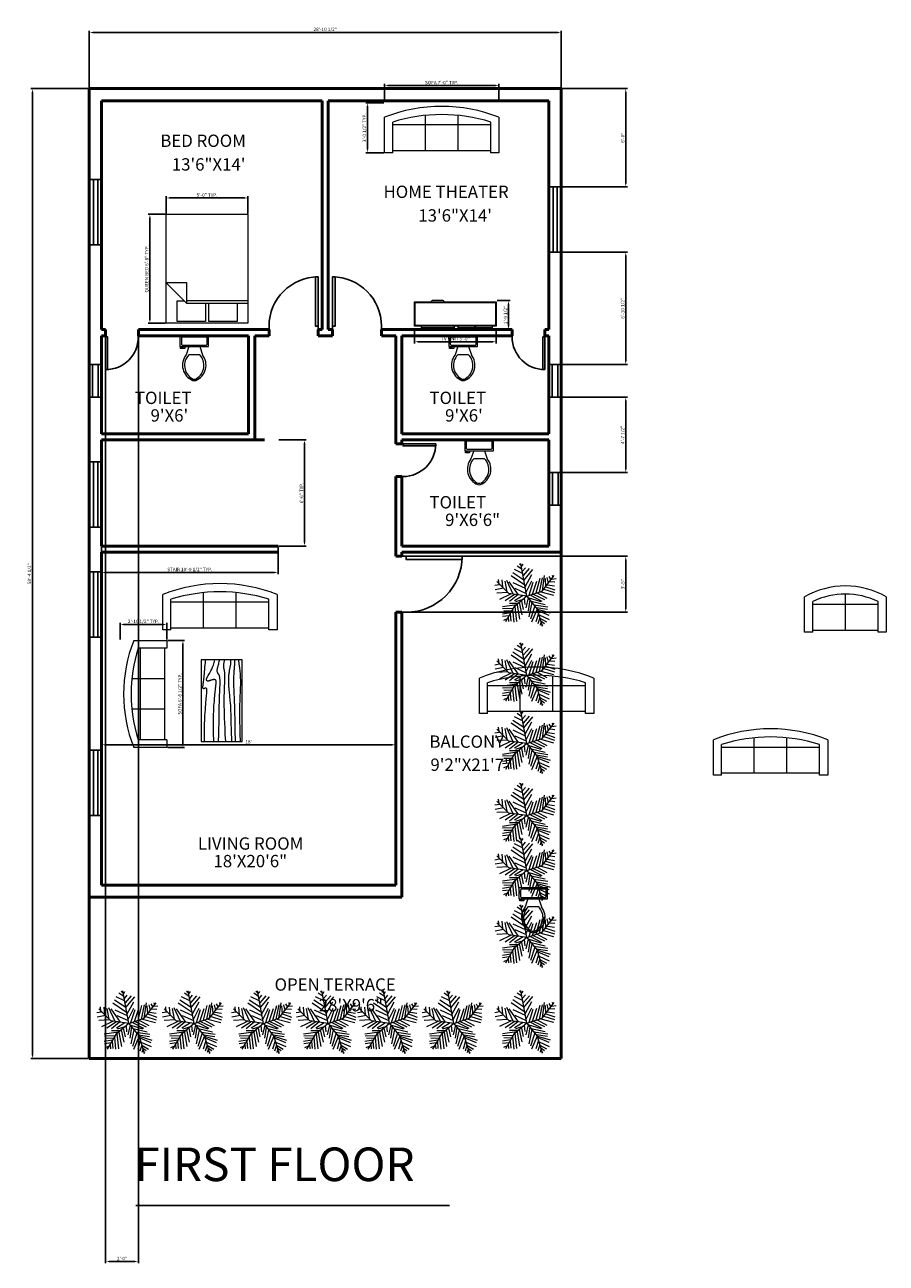
# Model space of a CAD drawing. Units: inches. Extents: x 2691 to 8091, y 3734 to 9067.
# Tile 5 of 5: x 3812 to 4444, y 3735 to 4645. Entities that reach past the tile are written whole.
import ezdxf

# ---------------------------------------------------------------- set-up
doc = ezdxf.new("R2010")
doc.units = ezdxf.units.IN
doc.layers.get('0').update_dxf_attribs({"color": 80})
for name, color, linetype, lineweight in [('A-ANNO-DIMS', 2, 'Continuous', 18), ('A-ANNO-TEXT', 7, 'Continuous', 25), ('A-AREA-IDEN', 7, 'Continuous', 18), ('A-FLOR-FIXT', 9, 'Continuous', 18), ('A-FURN', 8, 'Continuous', 18), ('A-WALL', 50, 'Continuous', 50), ('doors', 10, 'Continuous', 25), ('L-PLNT', 80, 'Continuous', 13), ('window', 4, 'Continuous', 25)]:
    doc.layers.add(name, color=color, linetype=linetype, lineweight=lineweight)
doc.styles.get("Standard").update_dxf_attribs({"font": 'arial.ttf'})
doc.dimstyles.new('ISO-25', dxfattribs={"dimtxt": 2.5, "dimasz": 2.5, "dimexe": 1.25, "dimexo": 0.625, "dimtad": 1, "dimdec": 1, "dimlunit": 3, "dimtxsty": 'Standard', "dimcen": 2.5, "dimadec": 0, "dimazin": 0, "dimtfac": 1, "dimtdec": 1, "dimtmove": 0, "dimatfit": 3, "dimfxl": 1, "dimarcsym": 0})

# ---------------------------------------------------------------- blocks, each defined once
blk = doc.blocks.new('Sofa - Roundback 7 ft.')
for p, q in [((-12.00002, -32.4421), (-12.00003, -6.5971)), ((11.99997, -32.4421), (11.99998, -6.5971)), ((-36.000027, -34), (-36.000027, -11.4696)), ((-35.999844, -13.3819), (35.9998, -13.3819)), ((35.99998, -34), (35.99998, -11.4696)), ((-36.000027, -32.4421), (35.99998, -32.4421))]:
    blk.add_line(p, q)
for points in [[(-36.000027, -34), (-42.000027, -34), (-42.000027, -8)], [(41.99998, -8), (41.99998, -34), (35.99998, -34)]]:
    blk.add_lwpolyline(points)
for centre, radius, start, end in [((0, -114.25), 114.25, 68.43141, 111.5686), ((-0.00001, -127.1968), 121.1968, 72.72033, 107.2797)]:
    blk.add_arc(centre, radius, start, end)
blk = doc.blocks.new('Toilet - top')
for p, q in [((-10, -8.5), (-8, -8.5)), ((-10, -9.5), (-10, -8.5)), ((-8, -8.5), (-8, -8)), ((-7, -8), (-7, -9.5)), ((-4, -8), (-6, -14)), ((4, -8), (6, -14)), ((9.5, -6), (9.5, -2)), ((-7, -9.5), (-10, -9.5)), ((4, -14), (-4, -14))]:
    blk.add_line(p, q)
blk.add_lwpolyline([(10.5, -8), (10.5, 0), (-10.5, 0), (-10.5, -8)], close=True)
for points in [[(-9.5, -2), (-9.5, -6)], [(8.5, -1), (-8.5, -1)], [(-8.5, -7), (8.5, -7)]]:
    blk.add_lwpolyline(points)
for centre, radius, start, end in [((-8.62, -1.88), 0.884, 81.8699, 188.1301), ((-8.62, -6.12), 0.884, 171.8699, 278.1301), ((8.62, -1.88), 0.884, 351.8699, 98.1301), ((8.62, -6.12), 0.884, 261.8699, 8.1301), ((3.52, -21.58), 12.17, 141.46911, 247.97143), ((4.2, -21.82), 11.33, 136.36773, 238.94682), ((-3.52, -21.58), 12.17, 292.02843, 38.53071), ((-4.2, -21.82), 11.33, 301.05301, 43.63209), ((0, -27.88), 4, 245.73182, 294.26817), ((0, -29), 4, 254.86053, 285.13947)]:
    blk.add_arc(centre, radius, start, end)
blk = doc.blocks.new('Sofa - Roundback Loveseat 5 ft.')
for p, q in [((0, -32.44198), (0, -5.99998)), ((-24, -33.99998), (-24, -11.46958)), ((-23.9998, -13.38178), (23.99986, -13.38178)), ((24.00004, -33.99998), (24.00004, -11.46958)), ((-24, -32.44198), (24.00004, -32.44198))]:
    blk.add_line(p, q)
for points in [[(-24, -33.99998), (-30, -33.99998), (-30, -7.99998)], [(30.00004, -7.99998), (30.00004, -33.99998), (24.00004, -33.99998)]]:
    blk.add_lwpolyline(points)
for centre, radius, start, end in [((0, -60.24998), 60.24998, 60.13715, 119.8628), ((0, -61.38438), 55.38444, 64.32083, 115.6792)]:
    blk.add_arc(centre, radius, start, end)
blk = doc.blocks.new('Bed - Queen')
for p, q in [((0, -80.00003), (0, 0)), ((0, 0), (59.99999, 0)), ((59.99999, 0), (59.99999, -80.00003)), ((7.99999, -1.2), (28.79998, -1.2)), ((7.99999, -14.4), (7.99999, -1.2)), ((28.79998, -1.2), (28.79998, -14.4)), ((31.19999, -1.2), (51.99999, -1.2)), ((31.19999, -14.4), (31.19999, -1.2)), ((51.99999, -1.2), (51.99999, -16.4)), ((0, -14.4), (44.8, -14.4)), ((44.8, -16.8), (0, -16.8)), ((59.99999, -29.6), (44.8, -14.4)), ((44.8, -14.4), (44.8, -29.6)), ((51.99999, -16.4), (46.79936, -16.4)), ((44.8, -29.6), (59.99999, -29.6)), ((59.99999, -80.00003), (0, -80.00003))]:
    blk.add_line(p, q)
blk = doc.blocks.new('Dining Set - 36 x 72 in')
at = {"layer": 'window'}
for p, q in [((418.4, 887.02), (466.4, 887.02)), ((418.4, 883.92), (466.4, 883.92))]:
    blk.add_line(p, q, dxfattribs=at)
blk.add_lwpolyline([(418.4, 881.14), (418.4, 890.14), (466.4, 890.14), (466.4, 881.14)], close=True, dxfattribs=at)
blk = doc.blocks.new('Table - Rectangular Woodgrain 60 x 30 in.')
for p, q in [((0, 0), (0, -30)), ((60, 0), (0, 0)), ((60, -30), (60, 0)), ((0, -30), (60, -30))]:
    blk.add_line(p, q)
for points in [[(0, -2.4), (4.8155, -2.418), (9.0302, -2.4688), (12.709, -2.5477), (15.9167, -2.65), (18.7181, -2.7711), (21.1781, -2.9063), (23.3616, -3.0508), (25.3333, -3.2), (27.1477, -3.3495), (28.8172, -3.4958), (30.3437, -3.636), (31.7291, -3.7667), (32.9756, -3.8849), (34.0849, -3.9875), (35.059, -4.0714), (35.9, -4.1334), (36.6114, -4.1711), (37.2041, -4.1854), (37.6906, -4.1779), (38.0833, -4.15), (38.3948, -4.1034), (38.6375, -4.0396), (38.8239, -3.9602), (38.9666, -3.8667), (39.0764, -3.7608), (39.1573, -3.6448), (39.2116, -3.521), (39.2416, -3.3917), (39.2498, -3.2593), (39.2385, -3.1261), (39.21, -2.9944), (39.1666, -2.8667), (39.111, -2.7447), (39.0468, -2.6281), (38.978, -2.5163), (38.9083, -2.4083), (38.8418, -2.3035), (38.7823, -2.201), (38.7337, -2.1001), (38.7, -2), (38.6844, -1.9003), (38.6875, -1.8021), (38.7094, -1.707), (38.75, -1.6167), (38.8094, -1.5326), (38.8875, -1.4563), (38.9844, -1.3893), (39.1, -1.3333), (39.2351, -1.2896), (39.3937, -1.2583), (39.5804, -1.2396), (39.8, -1.2333), (40.057, -1.2396), (40.3562, -1.2583), (40.7023, -1.2896), (41.1, -1.3333), (41.5547, -1.3895), (42.0755, -1.4573), (42.6721, -1.5361), (43.3542, -1.625), (44.1316, -1.7233), (45.014, -1.8302), (46.0114, -1.9449), (47.1333, -2.0667), (48.3862, -2.1947), (49.7625, -2.3281), (51.2513, -2.4663), (52.8416, -2.6083), (54.5226, -2.7535), (56.2833, -2.9011), (58.1127, -3.0501), (60, -3.2)], [(0, -9.2), (6.5759, -9.0858), (11.9385, -9.0365), (16.2527, -9.0418), (19.6833, -9.0917), (22.3952, -9.1759), (24.5531, -9.2844), (26.322, -9.4069), (27.8666, -9.5333), (29.3241, -9.6553), (30.7203, -9.7719), (32.0532, -9.8837), (33.3208, -9.9917), (34.5213, -10.0965), (35.6526, -10.199), (36.7128, -10.2999), (37.7, -10.4), (38.6129, -10.4996), (39.4531, -10.5969), (40.223, -10.6895), (40.925, -10.775), (41.5613, -10.8512), (42.1344, -10.9156), (42.6465, -10.966), (43.1, -11), (43.4976, -11.0158), (43.8437, -11.0136), (44.143, -10.9942), (44.4, -10.9583), (44.6195, -10.9069), (44.8062, -10.8406), (44.9648, -10.7603), (45.1, -10.6667), (45.2155, -10.5598), (45.3114, -10.4365), (45.3871, -10.2929), (45.4416, -10.125), (45.4743, -9.929), (45.4844, -9.7011), (45.4709, -9.4371), (45.4333, -9.1333), (45.3716, -8.7883), (45.2896, -8.4104), (45.1919, -8.0107), (45.0833, -7.6), (44.9685, -7.1893), (44.8521, -6.7896), (44.7388, -6.4117), (44.6333, -6.0667), (44.54, -5.7628), (44.4614, -5.4979), (44.4001, -5.2675), (44.3583, -5.0667), (44.3384, -4.8909), (44.3427, -4.7354), (44.3736, -4.5956), (44.4333, -4.4667), (44.5236, -4.3453), (44.6427, -4.2333), (44.7884, -4.1339), (44.9583, -4.05), (45.1501, -3.9849), (45.3614, -3.9417), (45.59, -3.9234), (45.8333, -3.9333), (46.0915, -3.9749), (46.3734, -4.0531), (46.6906, -4.1736), (47.0542, -4.3417), (47.4756, -4.5629), (47.9661, -4.8427), (48.5372, -5.1866), (49.2, -5.6), (49.9676, -6.0844), (50.8594, -6.625), (51.8965, -7.2031), (53.1, -7.8), (54.491, -8.3969), (56.0906, -8.975), (57.9199, -9.5156), (60, -10)], [(0, -12.8), (5.1847, -12.9322), (9.6213, -13.0323), (13.3963, -13.1059), (16.5958, -13.1583), (19.3063, -13.1952), (21.614, -13.2219), (23.6054, -13.2439), (25.3666, -13.2667), (26.9728, -13.2947), (28.4531, -13.3281), (29.8256, -13.3663), (31.1083, -13.4083), (32.3191, -13.4535), (33.476, -13.501), (34.597, -13.5501), (35.7, -13.6), (36.7984, -13.6497), (37.8875, -13.6979), (38.9578, -13.743), (40, -13.7833), (41.0047, -13.8174), (41.9625, -13.8438), (42.864, -13.8607), (43.7, -13.8667), (44.4631, -13.8604), (45.1552, -13.8417), (45.7801, -13.8104), (46.3416, -13.7667), (46.8439, -13.7104), (47.2906, -13.6417), (47.6858, -13.5604), (48.0333, -13.4667), (48.3375, -13.3608), (48.6042, -13.2448), (48.8396, -13.121), (49.05, -12.9917), (49.2417, -12.8593), (49.4208, -12.7261), (49.5937, -12.5944), (49.7667, -12.4667), (49.9452, -12.3451), (50.1323, -12.2313), (50.3303, -12.1268), (50.5416, -12.0333), (50.7686, -11.9524), (51.0135, -11.8854), (51.2788, -11.8341), (51.5666, -11.8), (51.8785, -11.7843), (52.2116, -11.7865), (52.562, -11.8059), (52.926, -11.8417), (53.2998, -11.8931), (53.6795, -11.9594), (54.0614, -12.0397), (54.4416, -12.1333), (54.8223, -12.2401), (55.2293, -12.3625), (55.6942, -12.5037), (56.2489, -12.6667), (56.9251, -12.8547), (57.7545, -13.0708), (58.7689, -13.3182), (60, -13.6)], [(0, -18), (5.124, -17.7273), (9.6609, -17.5057), (13.6705, -17.3303), (17.2125, -17.1958), (20.3467, -17.0973), (23.1328, -17.0297), (25.6307, -16.9878), (27.9, -16.9667), (29.9928, -16.9617), (31.9302, -16.9703), (33.7254, -16.9907), (35.3917, -17.0208), (36.9423, -17.0588), (38.3906, -17.1026), (39.7499, -17.1503), (41.0333, -17.2), (42.2519, -17.2496), (43.4073, -17.2969), (44.4986, -17.3395), (45.525, -17.375), (46.4858, -17.4012), (47.3802, -17.4156), (48.2074, -17.416), (48.9667, -17.4), (49.6583, -17.3662), (50.2872, -17.3167), (50.8595, -17.2547), (51.3812, -17.1833), (51.8584, -17.1057), (52.2971, -17.025), (52.7034, -16.9443), (53.0833, -16.8667), (53.443, -16.7951), (53.789, -16.7313), (54.128, -16.6768), (54.4666, -16.6334), (54.8115, -16.6024), (55.1693, -16.5854), (55.5465, -16.5841), (55.95, -16.6), (56.3828, -16.6337), (56.8346, -16.6823), (57.2915, -16.7418), (57.7396, -16.8084), (58.165, -16.878), (58.5539, -16.9469), (58.8924, -17.0111), (59.1666, -17.0667), (59.3679, -17.1107), (59.5078, -17.1438), (59.6032, -17.1675), (59.6708, -17.1833), (59.7275, -17.193), (59.7901, -17.1979), (59.8753, -17.1998), (60, -17.2)], [(0, -22.4), (8.0098, -22.2501), (14.4094, -22.1011), (19.4168, -21.9535), (23.25, -21.8083), (26.1269, -21.6663), (28.2656, -21.5281), (29.884, -21.3947), (31.2, -21.2667), (32.3967, -21.1448), (33.5172, -21.0292), (34.5697, -20.9198), (35.5625, -20.8167), (36.5037, -20.7198), (37.4015, -20.6292), (38.2642, -20.5448), (39.1, -20.4667), (39.9164, -20.3951), (40.7187, -20.3313), (41.5117, -20.2768), (42.3, -20.2333), (43.0883, -20.2024), (43.8812, -20.1854), (44.6836, -20.1841), (45.5, -20.2), (46.3328, -20.234), (47.1747, -20.2844), (48.0163, -20.3488), (48.8479, -20.425), (49.66, -20.5106), (50.4429, -20.6031), (51.1872, -20.7004), (51.8833, -20.8), (52.5246, -20.8999), (53.1166, -20.9995), (53.6681, -21.0983), (54.1875, -21.1958), (54.6834, -21.2919), (55.1646, -21.3859), (55.6394, -21.4777), (56.1167, -21.5667), (56.6028, -21.6515), (57.0961, -21.7266), (57.5929, -21.7852), (58.0896, -21.8208), (58.5823, -21.8268), (59.0674, -21.7964), (59.5412, -21.723), (60, -21.6)], [(0, -25.2), (8.6355, -25.0504), (15.7026, -24.9031), (21.4049, -24.7606), (25.9458, -24.625), (29.529, -24.4988), (32.3578, -24.3844), (34.6359, -24.284), (36.5667, -24.2), (38.3213, -24.1341), (39.9417, -24.0854), (41.437, -24.0523), (42.8167, -24.0333), (44.0901, -24.0268), (45.2667, -24.0313), (46.3557, -24.0451), (47.3667, -24.0667), (48.309, -24.0947), (49.1928, -24.1287), (50.0284, -24.168), (50.826, -24.2125), (51.5959, -24.2617), (52.3483, -24.3151), (53.0935, -24.3725), (53.8417, -24.4334), (54.6009, -24.497), (55.3699, -24.561), (56.1454, -24.6226), (56.9239, -24.6792), (57.7021, -24.7279), (58.4764, -24.7662), (59.2435, -24.7911), (60, -24.8)], [(0, -28.8), (5.6867, -28.6681), (10.45, -28.5698), (14.407, -28.5012), (17.675, -28.4584), (20.3711, -28.4374), (22.6125, -28.4344), (24.5164, -28.4455), (26.2, -28.4667), (27.762, -28.4947), (29.2276, -28.5281), (30.6033, -28.5663), (31.8958, -28.6084), (33.1118, -28.6535), (34.2578, -28.7011), (35.3405, -28.7501), (36.3666, -28.8), (37.3443, -28.8497), (38.288, -28.8974), (39.2137, -28.9412), (40.1375, -28.9792), (41.0753, -29.0093), (42.0432, -29.0297), (43.0572, -29.0384), (44.1333, -29.0333), (45.2936, -29.0114), (46.5843, -28.9641), (48.0579, -28.8816), (49.7666, -28.7542), (51.7629, -28.5721), (54.0989, -28.3255), (56.8272, -28.0048), (60, -27.6)]]:
    blk.add_lwpolyline(points)
blk = doc.blocks.new('new block')
at = {"layer": 'window'}
for p, q in [((-15.79, 35.68), (-15.79, 11.68)), ((-11.65, 35.68), (-11.65, 11.68))]:
    blk.add_line(p, q, dxfattribs=at)
blk.add_lwpolyline([(-9.22, 35.68), (-18.22, 35.68), (-18.22, 11.68), (-9.22, 11.68)], close=True, dxfattribs=at)
blk = doc.blocks.new('*U13')
for p, q in [((0, 0), (0, -100)), ((750, 0), (750, -100))]:
    blk.add_line(p, q)
blk.add_lwpolyline([(0, 0), (0, 750), (43.75, 750), (43.75, 0)], close=True)
blk.add_arc((0, 0), 750, 0, 90)
blk = doc.blocks.new('Entertainment Center')
for p, q in [((-4, 0), (-5, -1)), ((4, 0), (-4, 0)), ((5, -1), (4, 0)), ((-17, -19), (-17, -1)), ((-17, -1), (43, -1)), ((-16.5, -18.5), (-16.5, -1.5)), ((-16.5, -1.5), (42.5, -1.5)), ((42.5, -1.5), (42.5, -18.5)), ((43, -1), (43, -19)), ((43, -19), (-17, -19)), ((42.5, -18.5), (-16.5, -18.5)), ((-12, -20), (-12, -19)), ((12, -20), (-12, -20)), ((12, -19), (12, -20)), ((15, -20), (15, -19)), ((27, -20), (15, -20)), ((27, -19), (27, -20)), ((28, -20), (28, -19)), ((40, -20), (28, -20)), ((40, -19), (40, -20))]:
    blk.add_line(p, q)
blk.add_arc((0, 40), 61, 259.6111, 280.3889)
blk = doc.blocks.new('*D15')
at = {"layer": 'A-ANNO-DIMS', "color": 0, "lineweight": -2, "transparency": 16777216}
for p, q in [((3867.93, 4013.44), (3867.93, 4117.12)), ((3870.43, 4115.87), (4081.43, 4115.87)), ((4083.93, 4013.44), (4083.93, 4117.12))]:
    blk.add_line(p, q, dxfattribs=at)
at = {"layer": 'A-ANNO-DIMS', "color": 0, "transparency": 16777216}
for points in [[(3870.43, 4116.29), (3870.43, 4115.46), (3867.93, 4115.87)], [(4081.43, 4116.29), (4081.43, 4115.46), (4083.93, 4115.87)]]:
    blk.add_solid(points, dxfattribs=at)
at = {"layer": 'Defpoints', "color": 0, "transparency": 16777216}
for p in [(4083.93, 4115.87), (3867.93, 4012.82), (4083.93, 4012.82)]:
    blk.add_point(p, dxfattribs=at)
at = {"layer": 'A-ANNO-DIMS', "color": 0, "transparency": 16777216, "insert": (3975.93, 4117.78), "char_height": 2.5, "attachment_point": 5}
blk.add_mtext("18'", dxfattribs=at)
blk = doc.blocks.new('*U18')
for p, q in [((-7.288, 39.707), (-21.778, 46.673)), ((-8.737, 47.138), (-17.069, 52.711)), ((-10.186, 53.64), (-13.084, 55.962)), ((0, 0), (-10.5, 57)), ((-9.099, 51.782), (-6.563, 55.962)), ((-7.65, 43.423), (-2.578, 49.46)), ((-5.839, 35.992), (4.667, 48.067)), ((-5.114, 27.632), (10.463, 46.673)), ((-31.5, 4.5), (-52.5, 25.5)), ((-48.585, 21.131), (-49.309, 29.026)), ((-43.513, 28.561), (-42.427, 15.558)), ((-38.442, 26.239), (-34.819, 7.663)), ((-35.544, 28.097), (-24.314, 3.947)), ((-14.533, 2.09), (-30.834, 25.31)), ((-3.665, 19.273), (-27.574, 35.527)), ((-5.114, 28.097), (-24.676, 40.636)), ((-24.314, 23.917), (-2.941, 13.7)), ((-2.941, 16.486), (8.652, 37.85)), ((-1.129, 6.734), (9.014, 26.704)), ((3.942, 1.625), (11.187, 24.381)), ((10.101, 3.483), (17.708, 26.239)), ((16.259, 5.805), (23.142, 31.348)), ((22.055, 7.198), (27.489, 32.277)), ((27, 9), (48, 36)), ((27.127, 9.056), (31.112, 35.992)), ((31.836, 30.883), (32.561, 16.486)), ((35.096, 32.741), (37.27, 22.524)), ((38.719, 34.134), (41.979, 28.561)), ((40.53, 25.775), (48.862, 24.846)), ((43.791, 29.954), (51.036, 30.883)), ((44.153, 36.456), (45.239, 32.741)), ((-47.498, 19.737), (-55.83, 18.344)), ((-40.615, 13.7), (-55.105, 10.913)), ((-33.37, 6.269), (-52.207, 5.34)), ((-28.299, 3.483), (-47.86, -5.805)), ((-21.416, 3.018), (-38.079, -8.128)), ((0, 0), (-31.5, 4.5)), ((-15.982, 2.09), (-30.11, -9.521)), ((0, 0), (-22.5, -19.5)), ((-6.563, 1.161), (-21.416, -8.128)), ((-20.691, 13.7), (-1.129, 4.876)), ((0, 0), (27, 9)), ((0, 0), (18, -22.5)), ((6.478, 1.625), (26.04, -8.592)), ((11.187, 3.483), (30.749, -5.805)), ((18.07, 5.805), (35.096, -3.483)), ((24.229, 7.663), (46.688, 1.625)), ((29.662, 12.307), (48.137, 6.269)), ((33.285, 16.486), (48.862, 10.913)), ((36.183, 19.737), (48.137, 17.88)), ((-17.431, -15.094), (-42.789, -18.809)), ((-24.314, -21.596), (-42.427, -22.06)), ((-22.5, -19.5), (-37.5, -45)), ((-15.257, -12.772), (-30.11, -12.772)), ((-20.691, -18.345), (-17.793, -44.352)), ((-6.563, -5.805), (-19.967, -9.985)), ((-17.069, -15.094), (-12.721, -40.172)), ((-13.446, -11.378), (-8.737, -32.741)), ((-9.461, -8.592), (-6.201, -23.453)), ((-4.752, -3.483), (-3.665, -14.629)), ((2.493, -3.019), (-1.491, -20.202)), ((1.769, -2.555), (24.229, -9.521)), ((5.029, -6.27), (2.131, -25.775)), ((9.014, -11.378), (3.58, -35.992)), ((14.085, -16.951), (6.478, -40.172)), ((7.565, -9.056), (32.198, -14.629)), ((12.274, -15.094), (36.907, -18.809)), ((16.259, -19.738), (36.183, -22.989)), ((-28.299, -29.026), (-42.789, -31.348)), ((-30.834, -34.135), (-42.427, -35.528)), ((-34.457, -39.708), (-40.978, -42.494)), ((-26.849, -26.24), (-40.253, -25.775)), ((-32.646, -36.921), (-31.921, -44.352)), ((-29.023, -30.884), (-27.936, -43.887)), ((-25.038, -23.918), (-22.865, -45.281)), ((18.07, -22.524), (8.289, -45.745)), ((20.244, -30.419), (15.897, -44.816)), ((18, -22.5), (27, -52.5)), ((18.433, -22.524), (40.53, -29.026)), ((19.157, -25.311), (38.719, -33.206)), ((22.78, -37.85), (19.519, -48.532)), ((21.331, -32.741), (39.081, -40.636)), ((22.78, -38.314), (34.372, -44.816)), ((24.591, -45.745), (23.142, -50.854)), ((24.591, -43.423), (30.749, -47.603)), ((26.764, -49.925), (28.213, -50.854))]:
    blk.add_line(p, q)
blk = doc.blocks.new('*D25')
at = {"layer": 'A-ANNO-DIMS', "color": 0, "lineweight": -2, "transparency": 16777216}
for p, q in [((3914.77, 4505.48), (3902.15, 4505.48)), ((3903.4, 4502.98), (3903.4, 4427.98)), ((3914.77, 4425.48), (3902.15, 4425.48))]:
    blk.add_line(p, q, dxfattribs=at)
at = {"layer": 'A-ANNO-DIMS', "color": 0, "transparency": 16777216}
for points in [[(3902.98, 4502.98), (3903.81, 4502.98), (3903.4, 4505.48)], [(3902.98, 4427.98), (3903.81, 4427.98), (3903.4, 4425.48)]]:
    blk.add_solid(points, dxfattribs=at)
at = {"layer": 'Defpoints', "color": 0, "transparency": 16777216}
for p in [(3915.4, 4505.48), (3903.4, 4425.48), (3915.4, 4425.48)]:
    blk.add_point(p, dxfattribs=at)
at = {"layer": 'A-ANNO-DIMS', "color": 0, "transparency": 16777216, "insert": (3901.4, 4465.48), "char_height": 2.5, "attachment_point": 5, "rotation": 90}
blk.add_mtext('QUEEN BED 6\'-8" TYP.', dxfattribs=at)
blk = doc.blocks.new('*D26')
at = {"layer": 'A-ANNO-DIMS', "color": 0, "lineweight": -2, "transparency": 16777216}
for p, q in [((3915.4, 4506.1), (3915.4, 4518.73)), ((3972.9, 4517.48), (3917.9, 4517.48)), ((3975.4, 4506.1), (3975.4, 4518.73))]:
    blk.add_line(p, q, dxfattribs=at)
at = {"layer": 'A-ANNO-DIMS', "color": 0, "transparency": 16777216}
for points in [[(3917.9, 4517.89), (3917.9, 4517.06), (3915.4, 4517.48)], [(3972.9, 4517.89), (3972.9, 4517.06), (3975.4, 4517.48)]]:
    blk.add_solid(points, dxfattribs=at)
at = {"layer": 'Defpoints', "color": 0, "transparency": 16777216}
for p in [(3915.4, 4517.48), (3915.4, 4505.48), (3975.4, 4505.48)]:
    blk.add_point(p, dxfattribs=at)
at = {"layer": 'A-ANNO-DIMS', "color": 0, "transparency": 16777216, "insert": (3945.4, 4519.38), "char_height": 2.5, "attachment_point": 5}
blk.add_mtext('5\'-0" TYP.', dxfattribs=at)
blk = doc.blocks.new('*D27')
at = {"layer": 'A-ANNO-DIMS', "color": 0, "lineweight": -2, "transparency": 16777216}
for p, q in [((4075.75, 4588.05), (4075.75, 4601.27)), ((4078.25, 4600.02), (4157.25, 4600.02)), ((4159.75, 4588.05), (4159.75, 4601.27))]:
    blk.add_line(p, q, dxfattribs=at)
at = {"layer": 'A-ANNO-DIMS', "color": 0, "transparency": 16777216}
for points in [[(4078.25, 4600.44), (4078.25, 4599.61), (4075.75, 4600.02)], [(4157.25, 4600.44), (4157.25, 4599.61), (4159.75, 4600.02)]]:
    blk.add_solid(points, dxfattribs=at)
at = {"layer": 'Defpoints', "color": 0, "transparency": 16777216}
for p in [(4159.75, 4600.02), (4075.75, 4587.42), (4159.75, 4587.42)]:
    blk.add_point(p, dxfattribs=at)
at = {"layer": 'A-ANNO-DIMS', "color": 0, "transparency": 16777216, "insert": (4117.75, 4601.94), "char_height": 2.5, "attachment_point": 5}
blk.add_mtext('SOFA 7\'-0" TYP.', dxfattribs=at)
blk = doc.blocks.new('*D28')
at = {"layer": 'A-ANNO-DIMS', "color": 0, "lineweight": -2, "transparency": 16777216}
for p, q in [((4075.12, 4587.42), (4061.9, 4587.42)), ((4063.15, 4553.26), (4063.15, 4584.92)), ((4075.12, 4550.76), (4061.9, 4550.76))]:
    blk.add_line(p, q, dxfattribs=at)
at = {"layer": 'A-ANNO-DIMS', "color": 0, "transparency": 16777216}
for points in [[(4062.73, 4584.92), (4063.56, 4584.92), (4063.15, 4587.42)], [(4062.73, 4553.26), (4063.56, 4553.26), (4063.15, 4550.76)]]:
    blk.add_solid(points, dxfattribs=at)
at = {"layer": 'Defpoints', "color": 0, "transparency": 16777216}
for p in [(4063.15, 4587.42), (4075.75, 4587.42), (4075.75, 4550.76)]:
    blk.add_point(p, dxfattribs=at)
at = {"layer": 'A-ANNO-DIMS', "color": 0, "transparency": 16777216, "insert": (4061.23, 4569.09), "char_height": 2.5, "attachment_point": 5, "rotation": 90}
blk.add_mtext('3\'-0 1/2" TYP.', dxfattribs=at)
blk = doc.blocks.new('*D29')
at = {"layer": 'A-ANNO-DIMS', "color": 0, "lineweight": -2, "transparency": 16777216}
for p, q in [((3916.52, 4192.45), (3928.93, 4192.45)), ((3927.68, 4116.35), (3927.68, 4189.95)), ((3916.52, 4113.85), (3928.93, 4113.85))]:
    blk.add_line(p, q, dxfattribs=at)
at = {"layer": 'A-ANNO-DIMS', "color": 0, "transparency": 16777216}
for points in [[(3927.27, 4189.95), (3928.1, 4189.95), (3927.68, 4192.45)], [(3927.27, 4116.35), (3928.1, 4116.35), (3927.68, 4113.85)]]:
    blk.add_solid(points, dxfattribs=at)
at = {"layer": 'Defpoints', "color": 0, "transparency": 16777216}
for p in [(3915.89, 4192.45), (3927.68, 4192.45), (3915.89, 4113.85)]:
    blk.add_point(p, dxfattribs=at)
at = {"layer": 'A-ANNO-DIMS', "color": 0, "transparency": 16777216, "insert": (3925.77, 4153.15), "char_height": 2.5, "attachment_point": 5, "rotation": 90}
blk.add_mtext('SOFA 6\'-6 1/2" TYP.', dxfattribs=at)
blk = doc.blocks.new('*D30')
at = {"layer": 'A-ANNO-DIMS', "color": 0, "lineweight": -2, "transparency": 16777216}
for p, q in [((3881.58, 4193.08), (3881.58, 4205.49)), ((3913.39, 4204.24), (3884.08, 4204.24)), ((3915.89, 4193.08), (3915.89, 4205.49))]:
    blk.add_line(p, q, dxfattribs=at)
at = {"layer": 'A-ANNO-DIMS', "color": 0, "transparency": 16777216}
for points in [[(3884.08, 4204.66), (3884.08, 4203.82), (3881.58, 4204.24)], [(3913.39, 4204.66), (3913.39, 4203.82), (3915.89, 4204.24)]]:
    blk.add_solid(points, dxfattribs=at)
at = {"layer": 'Defpoints', "color": 0, "transparency": 16777216}
for p in [(3881.58, 4204.24), (3881.58, 4192.45), (3915.89, 4192.45)]:
    blk.add_point(p, dxfattribs=at)
at = {"layer": 'A-ANNO-DIMS', "color": 0, "transparency": 16777216, "insert": (3898.74, 4206.16), "char_height": 2.5, "attachment_point": 5}
blk.add_mtext('2\'-10 1/2" TYP.', dxfattribs=at)
blk = doc.blocks.new('*D39')
at = {"layer": 'A-ANNO-DIMS', "color": 0, "lineweight": -2, "transparency": 16777216}
for p, q in [((3867.93, 4261.19), (3867.93, 4241.13)), ((3997.53, 4261.19), (3997.53, 4241.13)), ((3870.43, 4242.38), (3995.03, 4242.38))]:
    blk.add_line(p, q, dxfattribs=at)
at = {"layer": 'A-ANNO-DIMS', "color": 0, "transparency": 16777216}
for points in [[(3870.43, 4242.8), (3870.43, 4241.96), (3867.93, 4242.38)], [(3995.03, 4242.8), (3995.03, 4241.96), (3997.53, 4242.38)]]:
    blk.add_solid(points, dxfattribs=at)
at = {"layer": 'Defpoints', "color": 0, "transparency": 16777216}
for p in [(3867.93, 4261.82), (3997.53, 4261.82), (3997.53, 4242.38)]:
    blk.add_point(p, dxfattribs=at)
at = {"layer": 'A-ANNO-DIMS', "color": 0, "transparency": 16777216, "insert": (3932.73, 4244.3), "char_height": 2.5, "attachment_point": 5}
blk.add_mtext('STAIR 10\'-9 1/2" TYP.', dxfattribs=at)
blk = doc.blocks.new('*D40')
at = {"layer": 'A-ANNO-DIMS', "color": 0, "lineweight": -2, "transparency": 16777216}
for p, q in [((3998.15, 4339.82), (4018.22, 4339.82)), ((4016.97, 4264.32), (4016.97, 4337.32)), ((3998.15, 4261.82), (4018.22, 4261.82))]:
    blk.add_line(p, q, dxfattribs=at)
at = {"layer": 'A-ANNO-DIMS', "color": 0, "transparency": 16777216}
for points in [[(4016.55, 4337.32), (4017.39, 4337.32), (4016.97, 4339.82)], [(4016.55, 4264.32), (4017.39, 4264.32), (4016.97, 4261.82)]]:
    blk.add_solid(points, dxfattribs=at)
at = {"layer": 'Defpoints', "color": 0, "transparency": 16777216}
for p in [(3997.53, 4339.82), (4016.97, 4339.82), (3997.53, 4261.82)]:
    blk.add_point(p, dxfattribs=at)
at = {"layer": 'A-ANNO-DIMS', "color": 0, "transparency": 16777216, "insert": (4015.07, 4300.82), "char_height": 2.5, "attachment_point": 5, "rotation": 90}
blk.add_mtext('6\'-6" TYP.', dxfattribs=at)
blk = doc.blocks.new('*D43')
at = {"layer": 'A-ANNO-DIMS', "color": 0, "lineweight": -2, "transparency": 16777216}
for p, q in [((4097.82, 4420.26), (4097.82, 4410.63)), ((4100.32, 4411.88), (4155.32, 4411.88)), ((4157.82, 4420.26), (4157.82, 4410.63))]:
    blk.add_line(p, q, dxfattribs=at)
at = {"layer": 'A-ANNO-DIMS', "color": 0, "transparency": 16777216}
for points in [[(4100.32, 4412.3), (4100.32, 4411.47), (4097.82, 4411.88)], [(4155.32, 4412.3), (4155.32, 4411.47), (4157.82, 4411.88)]]:
    blk.add_solid(points, dxfattribs=at)
at = {"layer": 'Defpoints', "color": 0, "transparency": 16777216}
for p in [(4097.82, 4420.88), (4157.82, 4420.88), (4157.82, 4411.88)]:
    blk.add_point(p, dxfattribs=at)
at = {"layer": 'A-ANNO-DIMS', "color": 0, "transparency": 16777216, "insert": (4127.82, 4413.78), "char_height": 2.5, "attachment_point": 5}
blk.add_mtext('TV UNIT 5\'-0"', dxfattribs=at)
blk = doc.blocks.new('*D44')
at = {"layer": 'A-ANNO-DIMS', "color": 0, "lineweight": -2, "transparency": 16777216}
for p, q in [((4158.45, 4442.22), (4168.07, 4442.22)), ((4166.82, 4423.38), (4166.82, 4439.72)), ((4158.45, 4420.88), (4168.07, 4420.88))]:
    blk.add_line(p, q, dxfattribs=at)
at = {"layer": 'A-ANNO-DIMS', "color": 0, "transparency": 16777216}
for points in [[(4166.4, 4439.72), (4167.24, 4439.72), (4166.82, 4442.22)], [(4166.4, 4423.38), (4167.24, 4423.38), (4166.82, 4420.88)]]:
    blk.add_solid(points, dxfattribs=at)
at = {"layer": 'Defpoints', "color": 0, "transparency": 16777216}
for p in [(4157.82, 4442.22), (4166.82, 4442.22), (4157.82, 4420.88)]:
    blk.add_point(p, dxfattribs=at)
at = {"layer": 'A-ANNO-DIMS', "color": 0, "transparency": 16777216, "insert": (4164.9, 4431.55), "char_height": 2.5, "attachment_point": 5, "rotation": 90}
blk.add_mtext('1\'-9 1/2"', dxfattribs=at)
blk = doc.blocks.new('*D51')
at = {"layer": 'A-ANNO-DIMS', "color": 0, "lineweight": -2, "transparency": 16777216}
for p, q in [((4206.06, 4597.82), (4254.16, 4597.82)), ((4252.91, 4528.21), (4252.91, 4595.32)), ((4206.06, 4525.71), (4254.16, 4525.71))]:
    blk.add_line(p, q, dxfattribs=at)
at = {"layer": 'A-ANNO-DIMS', "color": 0, "transparency": 16777216}
for points in [[(4252.5, 4595.32), (4253.33, 4595.32), (4252.91, 4597.82)], [(4252.5, 4528.21), (4253.33, 4528.21), (4252.91, 4525.71)]]:
    blk.add_solid(points, dxfattribs=at)
at = {"layer": 'Defpoints', "color": 0, "transparency": 16777216}
for p in [(4205.43, 4597.82), (4252.91, 4597.82), (4205.43, 4525.71)]:
    blk.add_point(p, dxfattribs=at)
at = {"layer": 'A-ANNO-DIMS', "color": 0, "transparency": 16777216, "insert": (4251.01, 4561.76), "char_height": 2.5, "attachment_point": 5, "rotation": 90}
blk.add_mtext('6\'-0"', dxfattribs=at)
blk = doc.blocks.new('*D52')
at = {"layer": 'A-ANNO-DIMS', "color": 0, "lineweight": -2, "transparency": 16777216}
for p, q in [((4206.06, 4477.71), (4254.16, 4477.71)), ((4252.91, 4397.72), (4252.91, 4475.21)), ((4206.06, 4395.22), (4254.16, 4395.22))]:
    blk.add_line(p, q, dxfattribs=at)
at = {"layer": 'A-ANNO-DIMS', "color": 0, "transparency": 16777216}
for points in [[(4252.5, 4475.21), (4253.33, 4475.21), (4252.91, 4477.71)], [(4252.5, 4397.72), (4253.33, 4397.72), (4252.91, 4395.22)]]:
    blk.add_solid(points, dxfattribs=at)
at = {"layer": 'Defpoints', "color": 0, "transparency": 16777216}
for p in [(4205.43, 4477.71), (4252.91, 4477.71), (4205.43, 4395.22)]:
    blk.add_point(p, dxfattribs=at)
at = {"layer": 'A-ANNO-DIMS', "color": 0, "transparency": 16777216, "insert": (4251, 4436.46), "char_height": 2.5, "attachment_point": 5, "rotation": 90}
blk.add_mtext('6\'-10 1/2"', dxfattribs=at)
blk = doc.blocks.new('*D53')
at = {"layer": 'A-ANNO-DIMS', "color": 0, "lineweight": -2, "transparency": 16777216}
for p, q in [((4206.06, 4371.22), (4254.16, 4371.22)), ((4252.91, 4318.29), (4252.91, 4368.72)), ((4206.26, 4315.79), (4254.16, 4315.79))]:
    blk.add_line(p, q, dxfattribs=at)
at = {"layer": 'A-ANNO-DIMS', "color": 0, "transparency": 16777216}
for points in [[(4252.5, 4368.72), (4253.33, 4368.72), (4252.91, 4371.22)], [(4252.5, 4318.29), (4253.33, 4318.29), (4252.91, 4315.79)]]:
    blk.add_solid(points, dxfattribs=at)
at = {"layer": 'Defpoints', "color": 0, "transparency": 16777216}
for p in [(4205.43, 4371.22), (4252.91, 4371.22), (4205.64, 4315.79)]:
    blk.add_point(p, dxfattribs=at)
at = {"layer": 'A-ANNO-DIMS', "color": 0, "transparency": 16777216, "insert": (4251, 4343.5), "char_height": 2.5, "attachment_point": 5, "rotation": 90}
blk.add_mtext('4\'-7 1/2"', dxfattribs=at)
blk = doc.blocks.new('*D60')
at = {"layer": 'A-ANNO-DIMS', "color": 0, "lineweight": -2, "transparency": 16777216}
for p, q in [((3870.93, 4420.19), (3870.93, 3735.06)), ((3894.93, 4420.19), (3894.93, 3735.06)), ((3873.43, 3736.31), (3892.43, 3736.31))]:
    blk.add_line(p, q, dxfattribs=at)
at = {"layer": 'A-ANNO-DIMS', "color": 0, "transparency": 16777216}
for points in [[(3873.43, 3736.72), (3873.43, 3735.89), (3870.93, 3736.31)], [(3892.43, 3736.72), (3892.43, 3735.89), (3894.93, 3736.31)]]:
    blk.add_solid(points, dxfattribs=at)
at = {"layer": 'Defpoints', "color": 0, "transparency": 16777216}
for p in [(3870.93, 4420.82), (3894.93, 4420.82), (3894.93, 3736.31)]:
    blk.add_point(p, dxfattribs=at)
at = {"layer": 'A-ANNO-DIMS', "color": 0, "transparency": 16777216, "insert": (3882.93, 3738.21), "char_height": 2.5, "attachment_point": 5}
blk.add_mtext('2\'-0"', dxfattribs=at)
blk = doc.blocks.new('*D61')
at = {"layer": 'A-ANNO-DIMS', "color": 0, "lineweight": -2, "transparency": 16777216}
for p, q in [((4089.06, 4254.32), (4254.16, 4254.32)), ((4252.91, 4215.82), (4252.91, 4251.82)), ((4089.06, 4213.32), (4254.16, 4213.32))]:
    blk.add_line(p, q, dxfattribs=at)
at = {"layer": 'A-ANNO-DIMS', "color": 0, "transparency": 16777216}
for points in [[(4252.5, 4251.82), (4253.33, 4251.82), (4252.91, 4254.32)], [(4252.5, 4215.82), (4253.33, 4215.82), (4252.91, 4213.32)]]:
    blk.add_solid(points, dxfattribs=at)
at = {"layer": 'Defpoints', "color": 0, "transparency": 16777216}
for p in [(4088.43, 4254.32), (4252.91, 4254.32), (4088.43, 4213.32)]:
    blk.add_point(p, dxfattribs=at)
at = {"layer": 'A-ANNO-DIMS', "color": 0, "transparency": 16777216, "insert": (4251.01, 4233.82), "char_height": 2.5, "attachment_point": 5, "rotation": 90}
blk.add_mtext('3\'-5"', dxfattribs=at)
blk = doc.blocks.new('*D69')
at = {"layer": 'A-ANNO-DIMS', "color": 0, "lineweight": -2, "transparency": 16777216}
for p, q in [((3858.93, 4598.44), (3858.93, 4640.32)), ((4205.43, 4598.44), (4205.43, 4640.32)), ((3861.43, 4639.07), (4202.93, 4639.07))]:
    blk.add_line(p, q, dxfattribs=at)
at = {"layer": 'A-ANNO-DIMS', "color": 0, "transparency": 16777216}
for points in [[(3861.43, 4639.49), (3861.43, 4638.65), (3858.93, 4639.07)], [(4202.93, 4639.49), (4202.93, 4638.65), (4205.43, 4639.07)]]:
    blk.add_solid(points, dxfattribs=at)
at = {"layer": 'Defpoints', "color": 0, "transparency": 16777216}
for p in [(4205.43, 4639.07), (3858.93, 4597.82), (4205.43, 4597.82)]:
    blk.add_point(p, dxfattribs=at)
at = {"layer": 'A-ANNO-DIMS', "color": 0, "transparency": 16777216, "insert": (4032.18, 4640.99), "char_height": 2.5, "attachment_point": 5}
blk.add_mtext('28\'-10 1/2"', dxfattribs=at)
blk = doc.blocks.new('*D70')
at = {"layer": 'A-ANNO-DIMS', "color": 0, "lineweight": -2, "transparency": 16777216}
for p, q in [((3858.31, 4597.82), (3815.91, 4597.82)), ((3817.16, 3887.82), (3817.16, 4595.32)), ((3858.31, 3885.32), (3815.91, 3885.32))]:
    blk.add_line(p, q, dxfattribs=at)
at = {"layer": 'A-ANNO-DIMS', "color": 0, "transparency": 16777216}
for points in [[(3816.75, 4595.32), (3817.58, 4595.32), (3817.16, 4597.82)], [(3816.75, 3887.82), (3817.58, 3887.82), (3817.16, 3885.32)]]:
    blk.add_solid(points, dxfattribs=at)
at = {"layer": 'Defpoints', "color": 0, "transparency": 16777216}
for p in [(3817.16, 4597.82), (3858.93, 4597.82), (3858.93, 3885.32)]:
    blk.add_point(p, dxfattribs=at)
at = {"layer": 'A-ANNO-DIMS', "color": 0, "transparency": 16777216, "insert": (3815.24, 4241.57), "char_height": 2.5, "attachment_point": 5, "rotation": 90}
blk.add_mtext('59\'-4 1/2"', dxfattribs=at)

msp = doc.modelspace()

# ---------------------------------------------------------------- linework, layer by layer
at = {"layer": 'A-ANNO-TEXT'}
msp.add_line((3893.15, 3777.56), (4123.54, 3777.56), dxfattribs=at)
at = {"layer": 'A-WALL'}
for p, q in [((3858.93, 4597.82), (3858.93, 3885.32)), ((3858.93, 4597.82), (4205.43, 4597.82)), ((4205.43, 4597.82), (4205.43, 3885.32)), ((3867.93, 4588.82), (3867.93, 4420.82)), ((3867.93, 4588.82), (4029.93, 4588.82)), ((4029.93, 4588.82), (4029.93, 4420.82)), ((4034.43, 4588.82), (4034.43, 4420.82)), ((4034.43, 4588.82), (4196.43, 4588.82)), ((4196.43, 4588.82), (4196.43, 4420.82)), ((3867.93, 4420.82), (3870.93, 4420.82)), ((3867.93, 4416.32), (3867.93, 4344.32)), ((3867.93, 4416.32), (3870.93, 4416.32)), ((3867.93, 4416.32), (3870.93, 4416.32)), ((3870.93, 4416.32), (3870.93, 4420.82)), ((3894.93, 4420.82), (3990.93, 4420.82)), ((3894.93, 4416.32), (3894.93, 4420.82)), ((3894.93, 4416.32), (3975.93, 4416.32)), ((3975.93, 4416.32), (3975.93, 4344.32)), ((3980.43, 4416.32), (3980.43, 4339.82)), ((3980.43, 4416.32), (3990.93, 4416.32)), ((3990.93, 4420.82), (3990.93, 4416.32)), ((4026.93, 4420.82), (4029.93, 4420.82)), ((4029.93, 4420.82), (4026.93, 4420.82)), ((4026.93, 4420.82), (4026.93, 4416.32)), ((4026.93, 4416.32), (4037.43, 4416.32)), ((4034.43, 4420.82), (4037.43, 4420.82)), ((4037.43, 4420.82), (4037.43, 4416.32)), ((4073.43, 4420.82), (4169.43, 4420.82)), ((4073.43, 4420.82), (4073.43, 4416.32)), ((4073.43, 4416.32), (4083.93, 4416.32)), ((4083.93, 4416.32), (4083.93, 4336.82)), ((4088.43, 4416.32), (4088.43, 4344.32)), ((4088.43, 4416.32), (4169.43, 4416.32)), ((4169.43, 4420.82), (4169.43, 4416.32)), ((4193.43, 4420.82), (4196.43, 4420.82)), ((4196.43, 4420.82), (4193.43, 4420.82)), ((4193.43, 4420.82), (4193.43, 4416.32)), ((4193.43, 4416.32), (4196.43, 4416.32)), ((4196.43, 4416.32), (4196.43, 4344.32)), ((3867.93, 4344.32), (3975.93, 4344.32)), ((3867.93, 4339.82), (3867.93, 4261.82)), ((3867.93, 4339.82), (3987.53, 4339.82)), ((4088.43, 4344.32), (4196.43, 4344.32)), ((4088.43, 4339.82), (4088.43, 4336.82)), ((4088.43, 4339.82), (4196.43, 4339.82)), ((4088.43, 4339.82), (4088.43, 4336.82)), ((4196.43, 4339.82), (4196.43, 4261.82)), ((4088.43, 4336.82), (4083.93, 4336.82)), ((4083.93, 4312.82), (4083.93, 4257.32)), ((4088.43, 4312.82), (4083.93, 4312.82)), ((4088.43, 4312.82), (4088.43, 4261.82)), ((3867.93, 4261.82), (3997.53, 4261.82)), ((3867.93, 4257.32), (3867.93, 4185.32)), ((3867.93, 4257.32), (3997.53, 4257.32)), ((4083.93, 4257.32), (4083.93, 4254.32)), ((4088.43, 4261.82), (4196.43, 4261.82)), ((4088.43, 4257.32), (4088.43, 4254.32)), ((4088.43, 4257.32), (4205.43, 4257.32)), ((4088.43, 4257.32), (4088.43, 4254.32)), ((4088.43, 4254.32), (4083.93, 4254.32)), ((4088.43, 4213.32), (4083.93, 4213.32)), ((4083.93, 4213.32), (4083.93, 4012.82)), ((4088.43, 4213.32), (4088.43, 4003.82)), ((3867.93, 4185.32), (3867.93, 4012.82)), ((3867.93, 4012.82), (4083.93, 4012.82)), ((4068.93, 4012.82), (4071.93, 4012.82)), ((4071.93, 4012.82), (4068.93, 4012.82)), ((3858.93, 4003.82), (4088.43, 4003.82)), ((3858.93, 3885.32), (4205.43, 3885.32))]:
    msp.add_line(p, q, dxfattribs=at)

# ---------------------------------------------------------------- block references
at = {"layer": 'A-FLOR-FIXT'}
for p in [(3936.01, 4416.32), (4133.54, 4416.32), (4145.24, 4339.87), (4185.01, 4010.74)]:
    msp.add_blockref('Toilet - top', p, dxfattribs=at)
at = {"layer": 'A-FURN'}
for name, p in [('Sofa - Roundback 7 ft.', (4117.75, 4584.76)), ('Entertainment Center', (4114.82, 4442.22)), ('Sofa - Roundback 7 ft.', (3954.89, 4234.22)), ('Sofa - Roundback Loveseat 5 ft.', (4414.23, 4232.52)), ('Sofa - Roundback 7 ft.', (4187.4, 4172.9)), ('Sofa - Roundback 7 ft.', (4359.31, 4127.59))]:
    msp.add_blockref(name, p, dxfattribs=at)
for name, p, rotation in [('Bed - Queen', (3975.4, 4425.48), 180), ('Table - Rectangular Woodgrain 60 x 30 in.', (3941.09, 4118.29), 90)]:
    msp.add_blockref(name, p, dxfattribs=dict(at, rotation=rotation))
at = {"layer": 'A-FURN', "xscale": 0.9357531878624332, "yscale": 0.9357531878624332, "zscale": 0.9357531878624332, "rotation": 90}
msp.add_blockref('Sofa - Roundback 7 ft.', (3884.08, 4153.15), dxfattribs=at)
at = {"layer": 'doors', "yscale": 0.0481264944431729, "zscale": 0.0481264944431729}
for p, xscale in [((4027.03, 4423.38), -0.0481264944431729), ((4037.43, 4423.38), 0.0481264944431729)]:
    msp.add_blockref('*U13', p, dxfattribs=dict(at, xscale=xscale))
at = {"layer": 'doors'}
for p, xscale, yscale, zscale, rotation in [((3870.93, 4415.38), -0.0319307598213287, 0.0319307598213287, 0.0319307598213287, 180), ((4193.43, 4415.38), 0.0319307598213287, 0.0319307598213287, 0.0319307598213287, 179.9999999999875), ((4089.38, 4336.82), 0.0319307598213287, 0.0319307598213287, 0.0319307598213287, 269.9999999999875), ((4091.66, 4254.32), 0.0547883317283913, 0.0547883317283913, 0.0547883317283913, 269.9999999999875)]:
    msp.add_blockref('*U13', p, dxfattribs=dict(at, xscale=xscale, yscale=yscale, zscale=zscale, rotation=rotation))
at = {"layer": 'L-PLNT', "xscale": 0.4200281787219986, "yscale": 0.4200281787219986, "zscale": 0.4200281787219986}
for p in [(4180.26, 4225.03), (4180.26, 4166.75), (4180.26, 4116.7), (4180.26, 4063.81), (4180.26, 4023.47), (4180.26, 3974.35), (3887.88, 3911.2), (3935.88, 3911.2), (3986.81, 3911.2), (4034.23, 3911.2), (4079.31, 3911.2), (4126.72, 3911.2), (4180.26, 3911.39)]:
    msp.add_blockref('*U18', p, dxfattribs=at)
at = {"layer": 'window', "rotation": 90}
for p in [(4749.07, 4064.6), (5086.57, 4059.31), (4749.07, 3857.27), (4749.07, 3776.49), (4749.07, 3645.45)]:
    msp.add_blockref('Dining Set - 36 x 72 in', p, dxfattribs=at)
at = {"layer": 'window'}
for p in [(3877.15, 4359.54), (4214.66, 4359.54), (4214.86, 4280.11)]:
    msp.add_blockref('new block', p, dxfattribs=at)

# ---------------------------------------------------------------- texts
at = {"layer": 'A-ANNO-TEXT'}
msp.add_text('FIRST FLOOR', height=24.6832, dxfattribs=at).set_placement((3891.98, 3795.36))
at = {"layer": 'A-AREA-IDEN'}
for s, height, p in [('BED ROOM', 9.054, (3911.05, 4554.99)), ('13\'6"X14\'', 9.054, (3919.52, 4537.63)), (' HOME THEATER', 9.0539, (4072.23, 4517.5)), ('13\'6"X14\'', 9.054, (4100.57, 4500.13)), ('TOILET', 9.054, (3892.44, 4366.16)), ('TOILET', 9.054, (4108.77, 4366.16)), ("9'X6'", 9.054, (3903.91, 4353.26)), ("9'X6'", 9.054, (4120.24, 4353.26)), ('TOILET', 9.054, (4108.77, 4289.46)), ('9\'X6\'6"', 9.054, (4120.24, 4276.56)), ('BALCONY', 9.054, (4108.73, 4113.64)), ('9\'2"X21\'7"', 9.054, (4109.46, 4096.7)), ('LIVING ROOM', 9.0539, (3938.65, 4038.81)), ('18\'X20\'6"', 9.054, (3950.12, 4025.91)), ('OPEN TERRACE', 9.0539, (3994.98, 3935.24)), ('28\'X9\'6"', 9.054, (4027.46, 3920.06))]:
    msp.add_text(s, height=height, dxfattribs=at).set_placement(p)

# ---------------------------------------------------------------- dimensions: what is measured, and where the dimension line sits
at = {"layer": 'A-ANNO-DIMS'}
for base, p1, p2, override, picture, middle in [((4205.43, 4639.07), (3858.93, 4597.82), (4205.43, 4597.82), {"dimdec": 1, "dimlfac": 1, "dimrnd": 0, "dimzin": 1, "dimdsep": 46, "dimlunit": 4, "dimfrac": 2}, '*D69', (4032.18, 4640.99)), ((3894.93, 3736.31), (3870.93, 4420.82), (3894.93, 4420.82), {"dimdec": 1, "dimlfac": 1, "dimrnd": 0, "dimzin": 1, "dimdsep": 46, "dimlunit": 4, "dimfrac": 2}, '*D60', (3882.93, 3738.21)), ((4083.93, 4115.87), (3867.93, 4012.82), (4083.93, 4012.82), {"dimclrd": 0, "dimclre": 0, "dimclrt": 0}, '*D15', (3975.93, 4117.78))]:
    dim = msp.add_linear_dim(base=base, p1=p1, p2=p2, dimstyle='ISO-25', override=override, dxfattribs=at)
    dim.commit()
    dim.dimension.update_dxf_attribs({"geometry": picture, "text_midpoint": middle})
for base, p1, p2, text, picture, middle in [((4159.75, 4600.02), (4075.75, 4587.42), (4159.75, 4587.42), 'SOFA <> TYP.', '*D27', (4117.75, 4601.94)), ((4157.82, 4411.88), (4097.82, 4420.88), (4157.82, 4420.88), 'TV UNIT <>', '*D43', (4127.82, 4413.78)), ((3997.53, 4242.38), (3867.93, 4261.82), (3997.53, 4261.82), 'STAIR <> TYP.', '*D39', (3932.73, 4244.3))]:
    dim = msp.add_linear_dim(base=base, p1=p1, p2=p2, text=text, dimstyle='ISO-25', override={"dimdec": 1, "dimlfac": 1, "dimrnd": 0, "dimzin": 1, "dimdsep": 46, "dimlunit": 4, "dimfrac": 2}, dxfattribs=at)
    dim.commit()
    dim.dimension.update_dxf_attribs({"geometry": picture, "text_midpoint": middle})
for base, p1, p2, picture, middle in [((3817.16, 4597.82), (3858.93, 3885.32), (3858.93, 4597.82), '*D70', (3815.24, 4241.57)), ((4252.91, 4597.82), (4205.43, 4525.71), (4205.43, 4597.82), '*D51', (4251.01, 4561.76)), ((4252.91, 4477.71), (4205.43, 4395.22), (4205.43, 4477.71), '*D52', (4251, 4436.46)), ((4166.82, 4442.22), (4157.82, 4420.88), (4157.82, 4442.22), '*D44', (4164.9, 4431.55)), ((4252.91, 4371.22), (4205.64, 4315.79), (4205.43, 4371.22), '*D53', (4251, 4343.5)), ((4252.91, 4254.32), (4088.43, 4213.32), (4088.43, 4254.32), '*D61', (4251.01, 4233.82))]:
    dim = msp.add_linear_dim(base=base, p1=p1, p2=p2, angle=90, dimstyle='ISO-25', override={"dimdec": 1, "dimlfac": 1, "dimrnd": 0, "dimzin": 1, "dimdsep": 46, "dimlunit": 4, "dimfrac": 2}, dxfattribs=at)
    dim.commit()
    dim.dimension.update_dxf_attribs({"geometry": picture, "text_midpoint": middle})
for base, p1, p2, angle, text, picture, middle in [((4063.15, 4587.42), (4075.75, 4550.76), (4075.75, 4587.42), 90, '<> TYP.', '*D28', (4061.23, 4569.09)), ((3915.4, 4517.48), (3975.4, 4505.48), (3915.4, 4505.48), 180, '<> TYP.', '*D26', (3945.4, 4519.38)), ((3903.4, 4425.48), (3915.4, 4505.48), (3915.4, 4425.48), 270, 'QUEEN BED <> TYP.', '*D25', (3901.4, 4465.48)), ((4016.97, 4339.82), (3997.53, 4261.82), (3997.53, 4339.82), 90, '<> TYP.', '*D40', (4015.07, 4300.82)), ((3881.58, 4204.24), (3915.89, 4192.45), (3881.58, 4192.45), 180, '<> TYP.', '*D30', (3898.74, 4206.16)), ((3927.68, 4192.45), (3915.89, 4113.85), (3915.89, 4192.45), 90, 'SOFA <> TYP.', '*D29', (3925.77, 4153.15))]:
    dim = msp.add_linear_dim(base=base, p1=p1, p2=p2, angle=angle, text=text, dimstyle='ISO-25', override={"dimdec": 1, "dimlfac": 1, "dimrnd": 0, "dimzin": 1, "dimdsep": 46, "dimlunit": 4, "dimfrac": 2}, dxfattribs=at)
    dim.commit()
    dim.dimension.update_dxf_attribs({"geometry": picture, "text_midpoint": middle})

doc.saveas('drawing.dxf')
